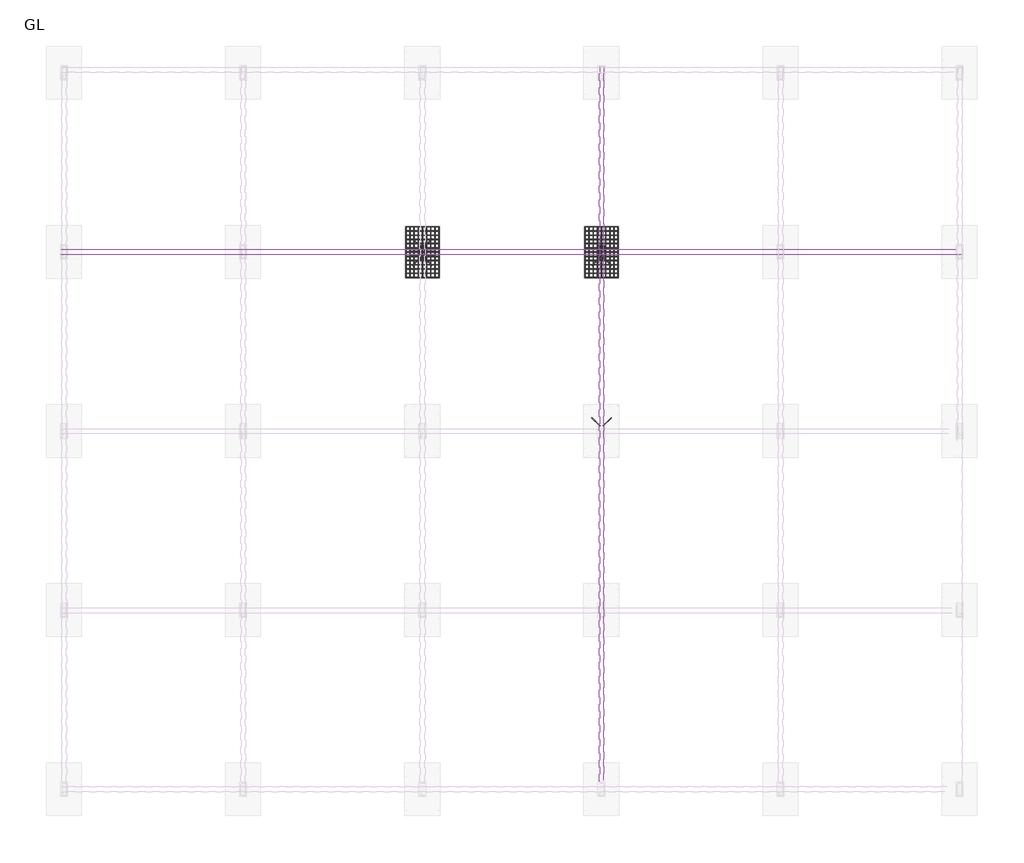
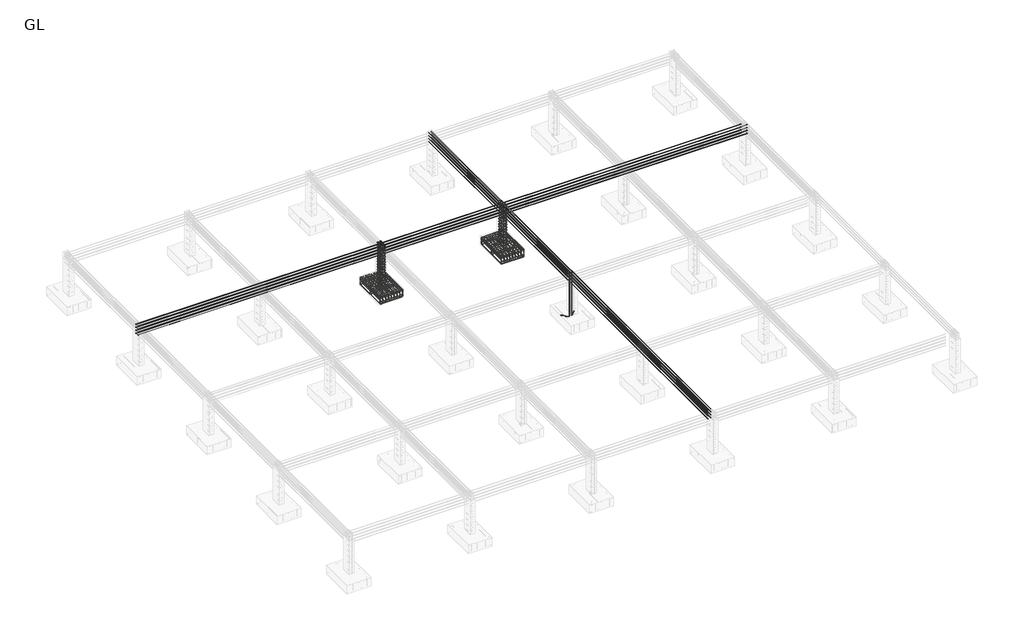
# One storey, part 9 of 16: 24 reinforcing bars.
"""IFC4 building model written with IfcOpenShell, lengths in millimetres."""

from ifc_helpers import new_model, si_unit, point, frame, origin, place, context, project, spatial, polyline, circle_curve, trimmed, segment, composite_curve, source, transform, mapped, element, save
from ifc_brep_helpers import swept_disk

model = new_model("IFC4")

# Units and contexts
model_context = context("Model", 3, world=origin())
ifc_project = project(units=[si_unit("LENGTHUNIT", "METRE", prefix="MILLI")], contexts=[model_context])

# Site, building, storey
site = spatial("IfcSite", under=ifc_project)
building = spatial("IfcBuilding", under=site)
storey = spatial("IfcBuildingStorey", under=building, Name="GL", Elevation=-1829.0)

# Reinforcing bars
placement = place(None, origin())
reinforcing_bar_shape = source(origin(), model_context, "Body", "SolidModel", [
    swept_disk(composite_curve([segment(polyline([(-3954.9544379, -1127.1167521, -2089.0), (-3954.9544379, -1127.1167521, -2213.0)]), True, "CONTINUOUS"), segment(trimmed(circle_curve(frame((-3984.9544379, -1127.1167521, -2213.0), z_axis=(0.0, 1.0, 0.0), x_axis=(30.0, 0.0, 0.0)), 30.0), [point((-3954.9544379, -1127.1167521, -2213.0))], [point((-3984.9544379, -1127.1167521, -2243.0))], True, "CARTESIAN"), True, "CONTINUOUS"), segment(polyline([(-3984.9544379, -1127.1167521, -2243.0), (-5052.9544379, -1127.1167521, -2243.0)]), True, "CONTINUOUS"), segment(trimmed(circle_curve(frame((-5052.9544379, -1127.1167521, -2213.0), z_axis=(0.0, 1.0, 0.0), x_axis=(0.0, 0.0, -30.0)), 30.0), [point((-5052.9544379, -1127.1167521, -2243.0))], [point((-5082.9544379, -1127.1167521, -2213.0))], True, "CARTESIAN"), True, "CONTINUOUS"), segment(polyline([(-5082.9544379, -1127.1167521, -2213.0), (-5082.9544379, -1127.1167521, -2089.0)]), True, "CONTINUOUS")], self_intersect=False), 6.0),
])
element("IfcReinforcingBar", 1, at=placement, inside=storey, context=model_context, shape_type="MappedRepresentation", body=[
    mapped(reinforcing_bar_shape, transform((0.0, 0.0, 0.0), x_axis=(1.0, 0.0, 0.0), y_axis=(0.0, 1.0, 0.0), z_axis=(0.0, 0.0, 1.0))),
    mapped(reinforcing_bar_shape, transform((0.0, -864.0, 0.0), x_axis=(1.0, 0.0, 0.0), y_axis=(0.0, 1.0, 0.0), z_axis=(0.0, 0.0, 1.0))),
    mapped(reinforcing_bar_shape, transform((0.0, -1728.0, 0.0), x_axis=(1.0, 0.0, 0.0), y_axis=(0.0, 1.0, 0.0), z_axis=(0.0, 0.0, 1.0))),
])
reinforcing_bar_2_shape = source(origin(), model_context, "Body", "SolidModel", [
    swept_disk(composite_curve([segment(polyline([(-5082.9544379, -1127.1167521, -2022.436678), (-5082.9544379, -1127.1167521, -1898.436678)]), True, "CONTINUOUS"), segment(trimmed(circle_curve(frame((-5052.9544379, -1127.1167521, -1898.436678), z_axis=(0.0, 1.0, 0.0), x_axis=(-30.0, 0.0, 0.0)), 30.0), [point((-5082.9544379, -1127.1167521, -1898.436678))], [point((-5052.9544379, -1127.1167521, -1868.436678))], True, "CARTESIAN"), True, "CONTINUOUS"), segment(polyline([(-5052.9544379, -1127.1167521, -1868.436678), (-3984.9544379, -1127.1167521, -1868.436678)]), True, "CONTINUOUS"), segment(trimmed(circle_curve(frame((-3984.9544379, -1127.1167521, -1898.436678), z_axis=(0.0, 1.0, 0.0), x_axis=(0.0, 0.0, 30.0)), 30.0), [point((-3984.9544379, -1127.1167521, -1868.436678))], [point((-3954.9544379, -1127.1167521, -1898.436678))], True, "CARTESIAN"), True, "CONTINUOUS"), segment(polyline([(-3954.9544379, -1127.1167521, -1898.436678), (-3954.9544379, -1127.1167521, -2022.436678)]), True, "CONTINUOUS")], self_intersect=False), 6.0),
])
element("IfcReinforcingBar", 2, at=placement, inside=storey, context=model_context, shape_type="MappedRepresentation", body=[
    mapped(reinforcing_bar_2_shape, transform((0.0, 0.0, 0.0), x_axis=(1.0, 0.0, 0.0), y_axis=(0.0, 1.0, 0.0), z_axis=(0.0, 0.0, 1.0))),
    mapped(reinforcing_bar_2_shape, transform((0.0, -144.0, 0.0), x_axis=(1.0, 0.0, 0.0), y_axis=(0.0, 1.0, 0.0), z_axis=(0.0, 0.0, 1.0))),
    mapped(reinforcing_bar_2_shape, transform((0.0, -288.0, 0.0), x_axis=(1.0, 0.0, 0.0), y_axis=(0.0, 1.0, 0.0), z_axis=(0.0, 0.0, 1.0))),
    mapped(reinforcing_bar_2_shape, transform((0.0, -432.0, 0.0), x_axis=(1.0, 0.0, 0.0), y_axis=(0.0, 1.0, 0.0), z_axis=(0.0, 0.0, 1.0))),
    mapped(reinforcing_bar_2_shape, transform((0.0, -576.0, 0.0), x_axis=(1.0, 0.0, 0.0), y_axis=(0.0, 1.0, 0.0), z_axis=(0.0, 0.0, 1.0))),
    mapped(reinforcing_bar_2_shape, transform((0.0, -720.0, 0.0), x_axis=(1.0, 0.0, 0.0), y_axis=(0.0, 1.0, 0.0), z_axis=(0.0, 0.0, 1.0))),
    mapped(reinforcing_bar_2_shape, transform((0.0, -864.0, 0.0), x_axis=(1.0, 0.0, 0.0), y_axis=(0.0, 1.0, 0.0), z_axis=(0.0, 0.0, 1.0))),
    mapped(reinforcing_bar_2_shape, transform((0.0, -1008.0, 0.0), x_axis=(1.0, 0.0, 0.0), y_axis=(0.0, 1.0, 0.0), z_axis=(0.0, 0.0, 1.0))),
    mapped(reinforcing_bar_2_shape, transform((0.0, -1152.0, 0.0), x_axis=(1.0, 0.0, 0.0), y_axis=(0.0, 1.0, 0.0), z_axis=(0.0, 0.0, 1.0))),
    mapped(reinforcing_bar_2_shape, transform((0.0, -1296.0, 0.0), x_axis=(1.0, 0.0, 0.0), y_axis=(0.0, 1.0, 0.0), z_axis=(0.0, 0.0, 1.0))),
    mapped(reinforcing_bar_2_shape, transform((0.0, -1440.0, 0.0), x_axis=(1.0, 0.0, 0.0), y_axis=(0.0, 1.0, 0.0), z_axis=(0.0, 0.0, 1.0))),
    mapped(reinforcing_bar_2_shape, transform((0.0, -1584.0, 0.0), x_axis=(1.0, 0.0, 0.0), y_axis=(0.0, 1.0, 0.0), z_axis=(0.0, 0.0, 1.0))),
    mapped(reinforcing_bar_2_shape, transform((0.0, -1728.0, 0.0), x_axis=(1.0, 0.0, 0.0), y_axis=(0.0, 1.0, 0.0), z_axis=(0.0, 0.0, 1.0))),
])
reinforcing_bar_3_shape = source(origin(), model_context, "Body", "SolidModel", [
    swept_disk(composite_curve([segment(polyline([(-5082.9544379, -2855.1167521, -2027.5081232), (-5082.9544379, -2855.1167521, -1903.5081232)]), True, "CONTINUOUS"), segment(trimmed(circle_curve(frame((-5082.9544379, -2825.1167521, -1903.5081232), z_axis=(-1.0, 0.0, 0.0), x_axis=(0.0, -30.0, 0.0)), 30.0), [point((-5082.9544379, -2855.1167521, -1903.5081232))], [point((-5082.9544379, -2825.1167521, -1873.5081232))], True, "CARTESIAN"), True, "CONTINUOUS"), segment(polyline([(-5082.9544379, -2825.1167521, -1873.5081232), (-5082.9544379, -1157.1167521, -1873.5081232)]), True, "CONTINUOUS"), segment(trimmed(circle_curve(frame((-5082.9544379, -1157.1167521, -1903.5081232), z_axis=(-1.0, 0.0, 0.0), x_axis=(0.0, 0.0, 30.0)), 30.0), [point((-5082.9544379, -1157.1167521, -1873.5081232))], [point((-5082.9544379, -1127.1167521, -1903.5081232))], True, "CARTESIAN"), True, "CONTINUOUS"), segment(polyline([(-5082.9544379, -1127.1167521, -1903.5081232), (-5082.9544379, -1127.1167521, -2027.5081232)]), True, "CONTINUOUS")], self_intersect=False), 6.0),
])
element("IfcReinforcingBar", 3, at=placement, inside=storey, context=model_context, shape_type="MappedRepresentation", body=[
    mapped(reinforcing_bar_3_shape, transform((0.0, 0.0, 0.0), x_axis=(1.0, 0.0, 0.0), y_axis=(0.0, 1.0, 0.0), z_axis=(0.0, 0.0, 1.0))),
    mapped(reinforcing_bar_3_shape, transform((141.0, 0.0, 0.0), x_axis=(1.0, 0.0, 0.0), y_axis=(0.0, 1.0, 0.0), z_axis=(0.0, 0.0, 1.0))),
    mapped(reinforcing_bar_3_shape, transform((282.0, 0.0, 0.0), x_axis=(1.0, 0.0, 0.0), y_axis=(0.0, 1.0, 0.0), z_axis=(0.0, 0.0, 1.0))),
    mapped(reinforcing_bar_3_shape, transform((423.0, 0.0, 0.0), x_axis=(1.0, 0.0, 0.0), y_axis=(0.0, 1.0, 0.0), z_axis=(0.0, 0.0, 1.0))),
    mapped(reinforcing_bar_3_shape, transform((564.0, 0.0, 0.0), x_axis=(1.0, 0.0, 0.0), y_axis=(0.0, 1.0, 0.0), z_axis=(0.0, 0.0, 1.0))),
    mapped(reinforcing_bar_3_shape, transform((705.0, 0.0, 0.0), x_axis=(1.0, 0.0, 0.0), y_axis=(0.0, 1.0, 0.0), z_axis=(0.0, 0.0, 1.0))),
    mapped(reinforcing_bar_3_shape, transform((846.0, 0.0, 0.0), x_axis=(1.0, 0.0, 0.0), y_axis=(0.0, 1.0, 0.0), z_axis=(0.0, 0.0, 1.0))),
    mapped(reinforcing_bar_3_shape, transform((987.0, 0.0, 0.0), x_axis=(1.0, 0.0, 0.0), y_axis=(0.0, 1.0, 0.0), z_axis=(0.0, 0.0, 1.0))),
    mapped(reinforcing_bar_3_shape, transform((1128.0, 0.0, 0.0), x_axis=(1.0, 0.0, 0.0), y_axis=(0.0, 1.0, 0.0), z_axis=(0.0, 0.0, 1.0))),
])
reinforcing_bar_4_shape = source(origin(), model_context, "Body", "SolidModel", [
    swept_disk(composite_curve([segment(polyline([(-3954.9544379, -2855.1167521, -2080.6239909), (-3954.9544379, -2855.1167521, -2204.6239909)]), True, "CONTINUOUS"), segment(trimmed(circle_curve(frame((-3954.9544379, -2825.1167521, -2204.6239909), z_axis=(1.0, 0.0, 0.0), x_axis=(0.0, -30.0, 0.0)), 30.0), [point((-3954.9544379, -2855.1167521, -2204.6239909))], [point((-3954.9544379, -2825.1167521, -2234.6239909))], True, "CARTESIAN"), True, "CONTINUOUS"), segment(polyline([(-3954.9544379, -2825.1167521, -2234.6239909), (-3954.9544379, -1170.1421892, -2234.6239909)]), True, "CONTINUOUS"), segment(trimmed(circle_curve(frame((-3954.9544379, -1170.1421892, -2204.6239909), z_axis=(1.0, 0.0, 0.0), x_axis=(0.0, 0.0, -30.0)), 30.0), [point((-3954.9544379, -1170.1421892, -2234.6239909))], [point((-3954.9544379, -1140.1421892, -2204.6239909))], True, "CARTESIAN"), True, "CONTINUOUS"), segment(polyline([(-3954.9544379, -1140.1421892, -2204.6239909), (-3954.9544379, -1140.1421892, -2080.6239909)]), True, "CONTINUOUS")], self_intersect=False), 6.0),
])
element("IfcReinforcingBar", 4, at=placement, inside=storey, context=model_context, shape_type="MappedRepresentation", body=[
    mapped(reinforcing_bar_4_shape, transform((0.0, 0.0, 0.0), x_axis=(1.0, 0.0, 0.0), y_axis=(0.0, 1.0, 0.0), z_axis=(0.0, 0.0, 1.0))),
    mapped(reinforcing_bar_4_shape, transform((-141.0, 0.0, 0.0), x_axis=(1.0, 0.0, 0.0), y_axis=(0.0, 1.0, 0.0), z_axis=(0.0, 0.0, 1.0))),
    mapped(reinforcing_bar_4_shape, transform((-282.0, 0.0, 0.0), x_axis=(1.0, 0.0, 0.0), y_axis=(0.0, 1.0, 0.0), z_axis=(0.0, 0.0, 1.0))),
    mapped(reinforcing_bar_4_shape, transform((-423.0, 0.0, 0.0), x_axis=(1.0, 0.0, 0.0), y_axis=(0.0, 1.0, 0.0), z_axis=(0.0, 0.0, 1.0))),
    mapped(reinforcing_bar_4_shape, transform((-564.0, 0.0, 0.0), x_axis=(1.0, 0.0, 0.0), y_axis=(0.0, 1.0, 0.0), z_axis=(0.0, 0.0, 1.0))),
    mapped(reinforcing_bar_4_shape, transform((-705.0, 0.0, 0.0), x_axis=(1.0, 0.0, 0.0), y_axis=(0.0, 1.0, 0.0), z_axis=(0.0, 0.0, 1.0))),
    mapped(reinforcing_bar_4_shape, transform((-846.0, 0.0, 0.0), x_axis=(1.0, 0.0, 0.0), y_axis=(0.0, 1.0, 0.0), z_axis=(0.0, 0.0, 1.0))),
    mapped(reinforcing_bar_4_shape, transform((-987.0, 0.0, 0.0), x_axis=(1.0, 0.0, 0.0), y_axis=(0.0, 1.0, 0.0), z_axis=(0.0, 0.0, 1.0))),
    mapped(reinforcing_bar_4_shape, transform((-1128.0, 0.0, 0.0), x_axis=(1.0, 0.0, 0.0), y_axis=(0.0, 1.0, 0.0), z_axis=(0.0, 0.0, 1.0))),
])
reinforcing_bar_5_shape = source(origin(), model_context, "Body", "SolidModel", [
    swept_disk(composite_curve([segment(polyline([(-10050.9544379, -1127.1167521, -2089.0), (-10050.9544379, -1127.1167521, -2213.0)]), True, "CONTINUOUS"), segment(trimmed(circle_curve(frame((-10080.9544379, -1127.1167521, -2213.0), z_axis=(0.0, 1.0, 0.0), x_axis=(30.0, 0.0, 0.0)), 30.0), [point((-10050.9544379, -1127.1167521, -2213.0))], [point((-10080.9544379, -1127.1167521, -2243.0))], True, "CARTESIAN"), True, "CONTINUOUS"), segment(polyline([(-10080.9544379, -1127.1167521, -2243.0), (-11148.9544379, -1127.1167521, -2243.0)]), True, "CONTINUOUS"), segment(trimmed(circle_curve(frame((-11148.9544379, -1127.1167521, -2213.0), z_axis=(0.0, 1.0, 0.0), x_axis=(0.0, 0.0, -30.0)), 30.0), [point((-11148.9544379, -1127.1167521, -2243.0))], [point((-11178.9544379, -1127.1167521, -2213.0))], True, "CARTESIAN"), True, "CONTINUOUS"), segment(polyline([(-11178.9544379, -1127.1167521, -2213.0), (-11178.9544379, -1127.1167521, -2089.0)]), True, "CONTINUOUS")], self_intersect=False), 6.0),
])
element("IfcReinforcingBar", 5, at=placement, inside=storey, context=model_context, shape_type="MappedRepresentation", body=[
    mapped(reinforcing_bar_5_shape, transform((0.0, 0.0, 0.0), x_axis=(1.0, 0.0, 0.0), y_axis=(0.0, 1.0, 0.0), z_axis=(0.0, 0.0, 1.0))),
    mapped(reinforcing_bar_5_shape, transform((0.0, -864.0, 0.0), x_axis=(1.0, 0.0, 0.0), y_axis=(0.0, 1.0, 0.0), z_axis=(0.0, 0.0, 1.0))),
    mapped(reinforcing_bar_5_shape, transform((0.0, -1728.0, 0.0), x_axis=(1.0, 0.0, 0.0), y_axis=(0.0, 1.0, 0.0), z_axis=(0.0, 0.0, 1.0))),
])
reinforcing_bar_6_shape = source(origin(), model_context, "Body", "SolidModel", [
    swept_disk(composite_curve([segment(polyline([(-11178.9544379, -1127.1167521, -2022.436678), (-11178.9544379, -1127.1167521, -1898.436678)]), True, "CONTINUOUS"), segment(trimmed(circle_curve(frame((-11148.9544379, -1127.1167521, -1898.436678), z_axis=(0.0, 1.0, 0.0), x_axis=(-30.0, 0.0, 0.0)), 30.0), [point((-11178.9544379, -1127.1167521, -1898.436678))], [point((-11148.9544379, -1127.1167521, -1868.436678))], True, "CARTESIAN"), True, "CONTINUOUS"), segment(polyline([(-11148.9544379, -1127.1167521, -1868.436678), (-10080.9544379, -1127.1167521, -1868.436678)]), True, "CONTINUOUS"), segment(trimmed(circle_curve(frame((-10080.9544379, -1127.1167521, -1898.436678), z_axis=(0.0, 1.0, 0.0), x_axis=(0.0, 0.0, 30.0)), 30.0), [point((-10080.9544379, -1127.1167521, -1868.436678))], [point((-10050.9544379, -1127.1167521, -1898.436678))], True, "CARTESIAN"), True, "CONTINUOUS"), segment(polyline([(-10050.9544379, -1127.1167521, -1898.436678), (-10050.9544379, -1127.1167521, -2022.436678)]), True, "CONTINUOUS")], self_intersect=False), 6.0),
])
element("IfcReinforcingBar", 6, at=placement, inside=storey, context=model_context, shape_type="MappedRepresentation", body=[
    mapped(reinforcing_bar_6_shape, transform((0.0, 0.0, 0.0), x_axis=(1.0, 0.0, 0.0), y_axis=(0.0, 1.0, 0.0), z_axis=(0.0, 0.0, 1.0))),
    mapped(reinforcing_bar_6_shape, transform((0.0, -144.0, 0.0), x_axis=(1.0, 0.0, 0.0), y_axis=(0.0, 1.0, 0.0), z_axis=(0.0, 0.0, 1.0))),
    mapped(reinforcing_bar_6_shape, transform((0.0, -288.0, 0.0), x_axis=(1.0, 0.0, 0.0), y_axis=(0.0, 1.0, 0.0), z_axis=(0.0, 0.0, 1.0))),
    mapped(reinforcing_bar_6_shape, transform((0.0, -432.0, 0.0), x_axis=(1.0, 0.0, 0.0), y_axis=(0.0, 1.0, 0.0), z_axis=(0.0, 0.0, 1.0))),
    mapped(reinforcing_bar_6_shape, transform((0.0, -576.0, 0.0), x_axis=(1.0, 0.0, 0.0), y_axis=(0.0, 1.0, 0.0), z_axis=(0.0, 0.0, 1.0))),
    mapped(reinforcing_bar_6_shape, transform((0.0, -720.0, 0.0), x_axis=(1.0, 0.0, 0.0), y_axis=(0.0, 1.0, 0.0), z_axis=(0.0, 0.0, 1.0))),
    mapped(reinforcing_bar_6_shape, transform((0.0, -864.0, 0.0), x_axis=(1.0, 0.0, 0.0), y_axis=(0.0, 1.0, 0.0), z_axis=(0.0, 0.0, 1.0))),
    mapped(reinforcing_bar_6_shape, transform((0.0, -1008.0, 0.0), x_axis=(1.0, 0.0, 0.0), y_axis=(0.0, 1.0, 0.0), z_axis=(0.0, 0.0, 1.0))),
    mapped(reinforcing_bar_6_shape, transform((0.0, -1152.0, 0.0), x_axis=(1.0, 0.0, 0.0), y_axis=(0.0, 1.0, 0.0), z_axis=(0.0, 0.0, 1.0))),
    mapped(reinforcing_bar_6_shape, transform((0.0, -1296.0, 0.0), x_axis=(1.0, 0.0, 0.0), y_axis=(0.0, 1.0, 0.0), z_axis=(0.0, 0.0, 1.0))),
    mapped(reinforcing_bar_6_shape, transform((0.0, -1440.0, 0.0), x_axis=(1.0, 0.0, 0.0), y_axis=(0.0, 1.0, 0.0), z_axis=(0.0, 0.0, 1.0))),
    mapped(reinforcing_bar_6_shape, transform((0.0, -1584.0, 0.0), x_axis=(1.0, 0.0, 0.0), y_axis=(0.0, 1.0, 0.0), z_axis=(0.0, 0.0, 1.0))),
    mapped(reinforcing_bar_6_shape, transform((0.0, -1728.0, 0.0), x_axis=(1.0, 0.0, 0.0), y_axis=(0.0, 1.0, 0.0), z_axis=(0.0, 0.0, 1.0))),
])
reinforcing_bar_7_shape = source(origin(), model_context, "Body", "SolidModel", [
    swept_disk(composite_curve([segment(polyline([(-11178.9544379, -2855.1167521, -2027.5081232), (-11178.9544379, -2855.1167521, -1903.5081232)]), True, "CONTINUOUS"), segment(trimmed(circle_curve(frame((-11178.9544379, -2825.1167521, -1903.5081232), z_axis=(-1.0, 0.0, 0.0), x_axis=(0.0, -30.0, 0.0)), 30.0), [point((-11178.9544379, -2855.1167521, -1903.5081232))], [point((-11178.9544379, -2825.1167521, -1873.5081232))], True, "CARTESIAN"), True, "CONTINUOUS"), segment(polyline([(-11178.9544379, -2825.1167521, -1873.5081232), (-11178.9544379, -1157.1167521, -1873.5081232)]), True, "CONTINUOUS"), segment(trimmed(circle_curve(frame((-11178.9544379, -1157.1167521, -1903.5081232), z_axis=(-1.0, 0.0, 0.0), x_axis=(0.0, 0.0, 30.0)), 30.0), [point((-11178.9544379, -1157.1167521, -1873.5081232))], [point((-11178.9544379, -1127.1167521, -1903.5081232))], True, "CARTESIAN"), True, "CONTINUOUS"), segment(polyline([(-11178.9544379, -1127.1167521, -1903.5081232), (-11178.9544379, -1127.1167521, -2027.5081232)]), True, "CONTINUOUS")], self_intersect=False), 6.0),
])
element("IfcReinforcingBar", 7, at=placement, inside=storey, context=model_context, shape_type="MappedRepresentation", body=[
    mapped(reinforcing_bar_7_shape, transform((0.0, 0.0, 0.0), x_axis=(1.0, 0.0, 0.0), y_axis=(0.0, 1.0, 0.0), z_axis=(0.0, 0.0, 1.0))),
    mapped(reinforcing_bar_7_shape, transform((141.0, 0.0, 0.0), x_axis=(1.0, 0.0, 0.0), y_axis=(0.0, 1.0, 0.0), z_axis=(0.0, 0.0, 1.0))),
    mapped(reinforcing_bar_7_shape, transform((282.0, 0.0, 0.0), x_axis=(1.0, 0.0, 0.0), y_axis=(0.0, 1.0, 0.0), z_axis=(0.0, 0.0, 1.0))),
    mapped(reinforcing_bar_7_shape, transform((423.0, 0.0, 0.0), x_axis=(1.0, 0.0, 0.0), y_axis=(0.0, 1.0, 0.0), z_axis=(0.0, 0.0, 1.0))),
    mapped(reinforcing_bar_7_shape, transform((564.0, 0.0, 0.0), x_axis=(1.0, 0.0, 0.0), y_axis=(0.0, 1.0, 0.0), z_axis=(0.0, 0.0, 1.0))),
    mapped(reinforcing_bar_7_shape, transform((705.0, 0.0, 0.0), x_axis=(1.0, 0.0, 0.0), y_axis=(0.0, 1.0, 0.0), z_axis=(0.0, 0.0, 1.0))),
    mapped(reinforcing_bar_7_shape, transform((846.0, 0.0, 0.0), x_axis=(1.0, 0.0, 0.0), y_axis=(0.0, 1.0, 0.0), z_axis=(0.0, 0.0, 1.0))),
    mapped(reinforcing_bar_7_shape, transform((987.0, 0.0, 0.0), x_axis=(1.0, 0.0, 0.0), y_axis=(0.0, 1.0, 0.0), z_axis=(0.0, 0.0, 1.0))),
    mapped(reinforcing_bar_7_shape, transform((1128.0, 0.0, 0.0), x_axis=(1.0, 0.0, 0.0), y_axis=(0.0, 1.0, 0.0), z_axis=(0.0, 0.0, 1.0))),
])
reinforcing_bar_8_shape = source(origin(), model_context, "Body", "SolidModel", [
    swept_disk(composite_curve([segment(polyline([(-10050.9544379, -2855.1167521, -2080.6239909), (-10050.9544379, -2855.1167521, -2204.6239909)]), True, "CONTINUOUS"), segment(trimmed(circle_curve(frame((-10050.9544379, -2825.1167521, -2204.6239909), z_axis=(1.0, 0.0, 0.0), x_axis=(0.0, -30.0, 0.0)), 30.0), [point((-10050.9544379, -2855.1167521, -2204.6239909))], [point((-10050.9544379, -2825.1167521, -2234.6239909))], True, "CARTESIAN"), True, "CONTINUOUS"), segment(polyline([(-10050.9544379, -2825.1167521, -2234.6239909), (-10050.9544379, -1170.1421892, -2234.6239909)]), True, "CONTINUOUS"), segment(trimmed(circle_curve(frame((-10050.9544379, -1170.1421892, -2204.6239909), z_axis=(1.0, 0.0, 0.0), x_axis=(0.0, 0.0, -30.0)), 30.0), [point((-10050.9544379, -1170.1421892, -2234.6239909))], [point((-10050.9544379, -1140.1421892, -2204.6239909))], True, "CARTESIAN"), True, "CONTINUOUS"), segment(polyline([(-10050.9544379, -1140.1421892, -2204.6239909), (-10050.9544379, -1140.1421892, -2080.6239909)]), True, "CONTINUOUS")], self_intersect=False), 6.0),
])
element("IfcReinforcingBar", 8, at=placement, inside=storey, context=model_context, shape_type="MappedRepresentation", body=[
    mapped(reinforcing_bar_8_shape, transform((0.0, 0.0, 0.0), x_axis=(1.0, 0.0, 0.0), y_axis=(0.0, 1.0, 0.0), z_axis=(0.0, 0.0, 1.0))),
    mapped(reinforcing_bar_8_shape, transform((-141.0, 0.0, 0.0), x_axis=(1.0, 0.0, 0.0), y_axis=(0.0, 1.0, 0.0), z_axis=(0.0, 0.0, 1.0))),
    mapped(reinforcing_bar_8_shape, transform((-282.0, 0.0, 0.0), x_axis=(1.0, 0.0, 0.0), y_axis=(0.0, 1.0, 0.0), z_axis=(0.0, 0.0, 1.0))),
    mapped(reinforcing_bar_8_shape, transform((-423.0, 0.0, 0.0), x_axis=(1.0, 0.0, 0.0), y_axis=(0.0, 1.0, 0.0), z_axis=(0.0, 0.0, 1.0))),
    mapped(reinforcing_bar_8_shape, transform((-564.0, 0.0, 0.0), x_axis=(1.0, 0.0, 0.0), y_axis=(0.0, 1.0, 0.0), z_axis=(0.0, 0.0, 1.0))),
    mapped(reinforcing_bar_8_shape, transform((-705.0, 0.0, 0.0), x_axis=(1.0, 0.0, 0.0), y_axis=(0.0, 1.0, 0.0), z_axis=(0.0, 0.0, 1.0))),
    mapped(reinforcing_bar_8_shape, transform((-846.0, 0.0, 0.0), x_axis=(1.0, 0.0, 0.0), y_axis=(0.0, 1.0, 0.0), z_axis=(0.0, 0.0, 1.0))),
    mapped(reinforcing_bar_8_shape, transform((-987.0, 0.0, 0.0), x_axis=(1.0, 0.0, 0.0), y_axis=(0.0, 1.0, 0.0), z_axis=(0.0, 0.0, 1.0))),
    mapped(reinforcing_bar_8_shape, transform((-1128.0, 0.0, 0.0), x_axis=(1.0, 0.0, 0.0), y_axis=(0.0, 1.0, 0.0), z_axis=(0.0, 0.0, 1.0))),
])
reinforcing_bar_9_shape = source(origin(), model_context, "Body", "SolidModel", [
    swept_disk(composite_curve([segment(polyline([(-10607.4864005, -2066.2223078, -1793.0), (-10695.1676414, -2153.9035486, -1793.0)]), True, "CONTINUOUS"), segment(trimmed(circle_curve(frame((-10673.9544379, -2175.1167521, -1793.0), z_axis=(0.0, 0.0, 1.0), x_axis=(-21.21320349999951, 21.213203500000418, 0.0)), 30.0), [point((-10695.1676414, -2153.9035486, -1793.0))], [point((-10673.9544379, -2205.1167521, -1793.0))], True, "CARTESIAN"), True, "CONTINUOUS"), segment(polyline([(-10673.9544379, -2205.1167521, -1793.0), (-10555.9544379, -2205.1167521, -1793.0)]), True, "CONTINUOUS"), segment(trimmed(circle_curve(frame((-10555.9544379, -2175.1167521, -1793.0), z_axis=(0.0, 0.0, 1.0), x_axis=(0.0, -30.0, 0.0)), 30.0), [point((-10555.9544379, -2205.1167521, -1793.0))], [point((-10525.9544379, -2175.1167521, -1793.0))], True, "CARTESIAN"), True, "CONTINUOUS"), segment(polyline([(-10525.9544379, -2175.1167521, -1793.0), (-10525.9544379, -1807.1167521, -1793.0)]), True, "CONTINUOUS"), segment(trimmed(circle_curve(frame((-10555.8864962, -1807.1167521, -1795.0178916), z_axis=(-0.06726305234213417, 0.0, 0.9977352764083365), x_axis=(29.93205830000079, 0.0, 2.0178915999999845)), 30.0), [point((-10525.9544379, -1807.1167521, -1793.0))], [point((-10555.8864962, -1777.1167521, -1795.0178916))], True, "CARTESIAN"), True, "CONTINUOUS"), segment(polyline([(-10555.8864962, -1777.1167521, -1795.0178916), (-10674.0223796, -1777.1167521, -1802.9821084)]), True, "CONTINUOUS"), segment(trimmed(circle_curve(frame((-10674.0223796, -1807.1167521, -1802.9821084), z_axis=(-0.06726305234213417, 0.0, 0.9977352764083365), x_axis=(0.0, 30.0, 0.0)), 30.0), [point((-10674.0223796, -1777.1167521, -1802.9821084))], [point((-10703.9544379, -1807.1167521, -1805.0))], True, "CARTESIAN"), True, "CONTINUOUS"), segment(polyline([(-10703.9544379, -1807.1167521, -1805.0), (-10703.9544379, -2175.1167521, -1805.0)]), True, "CONTINUOUS"), segment(trimmed(circle_curve(frame((-10673.9544379, -2175.1167521, -1805.0), z_axis=(0.0, 0.0, 1.0), x_axis=(-30.0, 0.0, 0.0)), 30.0), [point((-10703.9544379, -2175.1167521, -1805.0))], [point((-10652.7412345, -2196.3299555, -1805.0))], True, "CARTESIAN"), True, "CONTINUOUS"), segment(polyline([(-10652.7412345, -2196.3299555, -1805.0), (-10565.0599936, -2108.6487146, -1805.0)]), True, "CONTINUOUS")], self_intersect=False), 6.0),
])
element("IfcReinforcingBar", 9, at=placement, inside=storey, context=model_context, shape_type="MappedRepresentation", body=[
    mapped(reinforcing_bar_9_shape, transform((0.0, 0.0, 0.0), x_axis=(1.0, 0.0, 0.0), y_axis=(0.0, 1.0, 0.0), z_axis=(0.0, 0.0, 1.0))),
    mapped(reinforcing_bar_9_shape, transform((0.0, 0.0, 144.8571429), x_axis=(1.0, 0.0, 0.0), y_axis=(0.0, 1.0, 0.0), z_axis=(0.0, 0.0, 1.0))),
    mapped(reinforcing_bar_9_shape, transform((0.0, 0.0, 289.7142857), x_axis=(1.0, 0.0, 0.0), y_axis=(0.0, 1.0, 0.0), z_axis=(0.0, 0.0, 1.0))),
    mapped(reinforcing_bar_9_shape, transform((0.0, 0.0, 434.5714286), x_axis=(1.0, 0.0, 0.0), y_axis=(0.0, 1.0, 0.0), z_axis=(0.0, 0.0, 1.0))),
    mapped(reinforcing_bar_9_shape, transform((0.0, 0.0, 579.4285714), x_axis=(1.0, 0.0, 0.0), y_axis=(0.0, 1.0, 0.0), z_axis=(0.0, 0.0, 1.0))),
    mapped(reinforcing_bar_9_shape, transform((0.0, 0.0, 724.2857143), x_axis=(1.0, 0.0, 0.0), y_axis=(0.0, 1.0, 0.0), z_axis=(0.0, 0.0, 1.0))),
    mapped(reinforcing_bar_9_shape, transform((0.0, 0.0, 869.1428571), x_axis=(1.0, 0.0, 0.0), y_axis=(0.0, 1.0, 0.0), z_axis=(0.0, 0.0, 1.0))),
    mapped(reinforcing_bar_9_shape, transform((0.0, 0.0, 1014.0), x_axis=(1.0, 0.0, 0.0), y_axis=(0.0, 1.0, 0.0), z_axis=(0.0, 0.0, 1.0))),
    mapped(reinforcing_bar_9_shape, transform((0.0, 0.0, 1158.8571429), x_axis=(1.0, 0.0, 0.0), y_axis=(0.0, 1.0, 0.0), z_axis=(0.0, 0.0, 1.0))),
    mapped(reinforcing_bar_9_shape, transform((0.0, 0.0, 1303.7142857), x_axis=(1.0, 0.0, 0.0), y_axis=(0.0, 1.0, 0.0), z_axis=(0.0, 0.0, 1.0))),
    mapped(reinforcing_bar_9_shape, transform((0.0, 0.0, 1448.5714286), x_axis=(1.0, 0.0, 0.0), y_axis=(0.0, 1.0, 0.0), z_axis=(0.0, 0.0, 1.0))),
    mapped(reinforcing_bar_9_shape, transform((0.0, 0.0, 1593.4285714), x_axis=(1.0, 0.0, 0.0), y_axis=(0.0, 1.0, 0.0), z_axis=(0.0, 0.0, 1.0))),
    mapped(reinforcing_bar_9_shape, transform((0.0, 0.0, 1738.2857143), x_axis=(1.0, 0.0, 0.0), y_axis=(0.0, 1.0, 0.0), z_axis=(0.0, 0.0, 1.0))),
    mapped(reinforcing_bar_9_shape, transform((0.0, 0.0, 1883.1428571), x_axis=(1.0, 0.0, 0.0), y_axis=(0.0, 1.0, 0.0), z_axis=(0.0, 0.0, 1.0))),
    mapped(reinforcing_bar_9_shape, transform((0.0, 0.0, 2028.0), x_axis=(1.0, 0.0, 0.0), y_axis=(0.0, 1.0, 0.0), z_axis=(0.0, 0.0, 1.0))),
])
element("IfcReinforcingBar", 10, at=placement, inside=storey, context=model_context, shape_type="SolidModel", body=[
    swept_disk(composite_curve([segment(polyline([(-10672.0642232, -2176.0642439, 241.0), (-10672.0642232, -2176.0642439, -2129.0)]), True, "CONTINUOUS"), segment(trimmed(circle_curve(frame((-10693.2774266, -2197.2774473, -2129.0), z_axis=(-0.7071067811865187, 0.7071067811865764, 0.0), x_axis=(21.213203400000566, 21.21320340000011, 0.0)), 30.0), [point((-10672.0642232, -2176.0642439, -2129.0))], [point((-10693.2774266, -2197.2774473, -2159.0))], True, "CARTESIAN"), True, "CONTINUOUS"), segment(polyline([(-10693.2774266, -2197.2774473, -2159.0), (-10940.7648, -2444.7648207, -2159.0)]), True, "CONTINUOUS")], self_intersect=False), 6.0),
])
element("IfcReinforcingBar", 11, at=placement, inside=storey, context=model_context, shape_type="SolidModel", body=[
    swept_disk(composite_curve([segment(polyline([(-10672.0642232, -1806.1692603, 241.0), (-10672.0642232, -1806.1692603, -2129.0)]), True, "CONTINUOUS"), segment(trimmed(circle_curve(frame((-10693.2774266, -1784.9560568, -2129.0), z_axis=(0.7071067811865218, 0.7071067811865733, 0.0), x_axis=(21.213203400000566, -21.213203499999963, 0.0)), 30.0), [point((-10672.0642232, -1806.1692603, -2129.0))], [point((-10693.2774266, -1784.9560568, -2159.0))], True, "CARTESIAN"), True, "CONTINUOUS"), segment(polyline([(-10693.2774266, -1784.9560568, -2159.0), (-10940.7648, -1537.4686834, -2159.0)]), True, "CONTINUOUS")], self_intersect=False), 6.0),
])
element("IfcReinforcingBar", 12, at=placement, inside=storey, context=model_context, shape_type="SolidModel", body=[
    swept_disk(composite_curve([segment(polyline([(-10557.8446527, -2176.0642439, 241.0), (-10557.8446527, -2176.0642439, -2129.0)]), True, "CONTINUOUS"), segment(trimmed(circle_curve(frame((-10536.6314492, -2197.2774473, -2129.0), z_axis=(-0.7071067811865248, -0.7071067811865703, 0.0), x_axis=(-21.21320349999951, 21.21320340000011, 0.0)), 30.0), [point((-10557.8446527, -2176.0642439, -2129.0))], [point((-10536.6314492, -2197.2774473, -2159.0))], True, "CARTESIAN"), True, "CONTINUOUS"), segment(polyline([(-10536.6314492, -2197.2774473, -2159.0), (-10289.1440758, -2444.7648207, -2159.0)]), True, "CONTINUOUS")], self_intersect=False), 6.0),
])
element("IfcReinforcingBar", 13, at=placement, inside=storey, context=model_context, shape_type="SolidModel", body=[
    swept_disk(composite_curve([segment(polyline([(-10557.8446527, -1806.1692603, 241.0), (-10557.8446527, -1806.1692603, -2129.0)]), True, "CONTINUOUS"), segment(trimmed(circle_curve(frame((-10536.6314492, -1784.9560568, -2129.0), z_axis=(0.7071067811865157, -0.7071067811865794, 0.0), x_axis=(-21.21320349999951, -21.213203499999963, 0.0)), 30.0), [point((-10557.8446527, -1806.1692603, -2129.0))], [point((-10536.6314492, -1784.9560568, -2159.0))], True, "CARTESIAN"), True, "CONTINUOUS"), segment(polyline([(-10536.6314492, -1784.9560568, -2159.0), (-10289.1440758, -1537.4686834, -2159.0)]), True, "CONTINUOUS")], self_intersect=False), 6.0),
])
reinforcing_bar_10_shape = source(origin(), model_context, "Body", "SolidModel", [
    swept_disk(composite_curve([segment(polyline([(-10672.0642232, -2098.9117405, 241.0), (-10672.0642232, -2098.9117405, -2129.0)]), True, "CONTINUOUS"), segment(trimmed(circle_curve(frame((-10702.0642232, -2098.9117405, -2129.0), z_axis=(0.0, 1.0, 0.0), x_axis=(30.0, 0.0, 0.0)), 30.0), [point((-10672.0642232, -2098.9117405, -2129.0))], [point((-10702.0642232, -2098.9117405, -2159.0))], True, "CARTESIAN"), True, "CONTINUOUS"), segment(polyline([(-10702.0642232, -2098.9117405, -2159.0), (-11052.0642232, -2098.9117405, -2159.0)]), True, "CONTINUOUS")], self_intersect=False), 6.0),
])
element("IfcReinforcingBar", 14, at=placement, inside=storey, context=model_context, shape_type="MappedRepresentation", body=[
    mapped(reinforcing_bar_10_shape, transform((0.0, 0.0, 0.0), x_axis=(1.0, 0.0, 0.0), y_axis=(0.0, 1.0, 0.0), z_axis=(0.0, 0.0, 1.0))),
    mapped(reinforcing_bar_10_shape, transform((0.0, 123.5823926, 0.0), x_axis=(1.0, 0.0, 0.0), y_axis=(0.0, 1.0, 0.0), z_axis=(0.0, 0.0, 1.0))),
    mapped(reinforcing_bar_10_shape, transform((0.0, 247.1647853, 0.0), x_axis=(1.0, 0.0, 0.0), y_axis=(0.0, 1.0, 0.0), z_axis=(0.0, 0.0, 1.0))),
])
reinforcing_bar_11_shape = source(origin(), model_context, "Body", "SolidModel", [
    swept_disk(composite_curve([segment(polyline([(-10557.8446527, -2098.9117405, 241.0), (-10557.8446527, -2098.9117405, -2129.0)]), True, "CONTINUOUS"), segment(trimmed(circle_curve(frame((-10527.8446527, -2098.9117405, -2129.0), z_axis=(0.0, -1.0, 0.0), x_axis=(-30.0, 0.0, 0.0)), 30.0), [point((-10557.8446527, -2098.9117405, -2129.0))], [point((-10527.8446527, -2098.9117405, -2159.0))], True, "CARTESIAN"), True, "CONTINUOUS"), segment(polyline([(-10527.8446527, -2098.9117405, -2159.0), (-10177.8446527, -2098.9117405, -2159.0)]), True, "CONTINUOUS")], self_intersect=False), 6.0),
])
element("IfcReinforcingBar", 15, at=placement, inside=storey, context=model_context, shape_type="MappedRepresentation", body=[
    mapped(reinforcing_bar_11_shape, transform((0.0, 0.0, 0.0), x_axis=(1.0, 0.0, 0.0), y_axis=(0.0, 1.0, 0.0), z_axis=(0.0, 0.0, 1.0))),
    mapped(reinforcing_bar_11_shape, transform((0.0, 123.5823926, 0.0), x_axis=(1.0, 0.0, 0.0), y_axis=(0.0, 1.0, 0.0), z_axis=(0.0, 0.0, 1.0))),
    mapped(reinforcing_bar_11_shape, transform((0.0, 247.1647853, 0.0), x_axis=(1.0, 0.0, 0.0), y_axis=(0.0, 1.0, 0.0), z_axis=(0.0, 0.0, 1.0))),
])
reinforcing_bar_12_shape = source(origin(), model_context, "Body", "SolidModel", [
    swept_disk(composite_curve([segment(polyline([(-4511.4864005, -2066.2223078, -1793.0), (-4599.1676414, -2153.9035486, -1793.0)]), True, "CONTINUOUS"), segment(trimmed(circle_curve(frame((-4577.9544379, -2175.1167521, -1793.0), z_axis=(0.0, 0.0, 1.0), x_axis=(-21.213203500000418, 21.213203500000418, 0.0)), 30.0), [point((-4599.1676414, -2153.9035486, -1793.0))], [point((-4577.9544379, -2205.1167521, -1793.0))], True, "CARTESIAN"), True, "CONTINUOUS"), segment(polyline([(-4577.9544379, -2205.1167521, -1793.0), (-4459.9544379, -2205.1167521, -1793.0)]), True, "CONTINUOUS"), segment(trimmed(circle_curve(frame((-4459.9544379, -2175.1167521, -1793.0), z_axis=(0.0, 0.0, 1.0), x_axis=(0.0, -30.0, 0.0)), 30.0), [point((-4459.9544379, -2205.1167521, -1793.0))], [point((-4429.9544379, -2175.1167521, -1793.0))], True, "CARTESIAN"), True, "CONTINUOUS"), segment(polyline([(-4429.9544379, -2175.1167521, -1793.0), (-4429.9544379, -1807.1167521, -1793.0)]), True, "CONTINUOUS"), segment(trimmed(circle_curve(frame((-4459.8864962, -1807.1167521, -1795.0178916), z_axis=(-0.06726305234213417, 0.0, 0.9977352764083365), x_axis=(29.93205829999988, 0.0, 2.0178915999999845)), 30.0), [point((-4429.9544379, -1807.1167521, -1793.0))], [point((-4459.8864962, -1777.1167521, -1795.0178916))], True, "CARTESIAN"), True, "CONTINUOUS"), segment(polyline([(-4459.8864962, -1777.1167521, -1795.0178916), (-4578.0223796, -1777.1167521, -1802.9821084)]), True, "CONTINUOUS"), segment(trimmed(circle_curve(frame((-4578.0223796, -1807.1167521, -1802.9821084), z_axis=(-0.06726305234213417, 0.0, 0.9977352764083365), x_axis=(0.0, 30.0, 0.0)), 30.0), [point((-4578.0223796, -1777.1167521, -1802.9821084))], [point((-4607.9544379, -1807.1167521, -1805.0))], True, "CARTESIAN"), True, "CONTINUOUS"), segment(polyline([(-4607.9544379, -1807.1167521, -1805.0), (-4607.9544379, -2175.1167521, -1805.0)]), True, "CONTINUOUS"), segment(trimmed(circle_curve(frame((-4577.9544379, -2175.1167521, -1805.0), z_axis=(0.0, 0.0, 1.0), x_axis=(-30.0, 0.0, 0.0)), 30.0), [point((-4607.9544379, -2175.1167521, -1805.0))], [point((-4556.7412345, -2196.3299555, -1805.0))], True, "CARTESIAN"), True, "CONTINUOUS"), segment(polyline([(-4556.7412345, -2196.3299555, -1805.0), (-4469.0599936, -2108.6487146, -1805.0)]), True, "CONTINUOUS")], self_intersect=False), 6.0),
])
element("IfcReinforcingBar", 16, at=placement, inside=storey, context=model_context, shape_type="MappedRepresentation", body=[
    mapped(reinforcing_bar_12_shape, transform((0.0, 0.0, 0.0), x_axis=(1.0, 0.0, 0.0), y_axis=(0.0, 1.0, 0.0), z_axis=(0.0, 0.0, 1.0))),
    mapped(reinforcing_bar_12_shape, transform((0.0, 0.0, 144.8571429), x_axis=(1.0, 0.0, 0.0), y_axis=(0.0, 1.0, 0.0), z_axis=(0.0, 0.0, 1.0))),
    mapped(reinforcing_bar_12_shape, transform((0.0, 0.0, 289.7142857), x_axis=(1.0, 0.0, 0.0), y_axis=(0.0, 1.0, 0.0), z_axis=(0.0, 0.0, 1.0))),
    mapped(reinforcing_bar_12_shape, transform((0.0, 0.0, 434.5714286), x_axis=(1.0, 0.0, 0.0), y_axis=(0.0, 1.0, 0.0), z_axis=(0.0, 0.0, 1.0))),
    mapped(reinforcing_bar_12_shape, transform((0.0, 0.0, 579.4285714), x_axis=(1.0, 0.0, 0.0), y_axis=(0.0, 1.0, 0.0), z_axis=(0.0, 0.0, 1.0))),
    mapped(reinforcing_bar_12_shape, transform((0.0, 0.0, 724.2857143), x_axis=(1.0, 0.0, 0.0), y_axis=(0.0, 1.0, 0.0), z_axis=(0.0, 0.0, 1.0))),
    mapped(reinforcing_bar_12_shape, transform((0.0, 0.0, 869.1428571), x_axis=(1.0, 0.0, 0.0), y_axis=(0.0, 1.0, 0.0), z_axis=(0.0, 0.0, 1.0))),
    mapped(reinforcing_bar_12_shape, transform((0.0, 0.0, 1014.0), x_axis=(1.0, 0.0, 0.0), y_axis=(0.0, 1.0, 0.0), z_axis=(0.0, 0.0, 1.0))),
    mapped(reinforcing_bar_12_shape, transform((0.0, 0.0, 1158.8571429), x_axis=(1.0, 0.0, 0.0), y_axis=(0.0, 1.0, 0.0), z_axis=(0.0, 0.0, 1.0))),
    mapped(reinforcing_bar_12_shape, transform((0.0, 0.0, 1303.7142857), x_axis=(1.0, 0.0, 0.0), y_axis=(0.0, 1.0, 0.0), z_axis=(0.0, 0.0, 1.0))),
    mapped(reinforcing_bar_12_shape, transform((0.0, 0.0, 1448.5714286), x_axis=(1.0, 0.0, 0.0), y_axis=(0.0, 1.0, 0.0), z_axis=(0.0, 0.0, 1.0))),
    mapped(reinforcing_bar_12_shape, transform((0.0, 0.0, 1593.4285714), x_axis=(1.0, 0.0, 0.0), y_axis=(0.0, 1.0, 0.0), z_axis=(0.0, 0.0, 1.0))),
    mapped(reinforcing_bar_12_shape, transform((0.0, 0.0, 1738.2857143), x_axis=(1.0, 0.0, 0.0), y_axis=(0.0, 1.0, 0.0), z_axis=(0.0, 0.0, 1.0))),
    mapped(reinforcing_bar_12_shape, transform((0.0, 0.0, 1883.1428571), x_axis=(1.0, 0.0, 0.0), y_axis=(0.0, 1.0, 0.0), z_axis=(0.0, 0.0, 1.0))),
    mapped(reinforcing_bar_12_shape, transform((0.0, 0.0, 2028.0), x_axis=(1.0, 0.0, 0.0), y_axis=(0.0, 1.0, 0.0), z_axis=(0.0, 0.0, 1.0))),
])
element("IfcReinforcingBar", 17, at=placement, inside=storey, context=model_context, shape_type="SolidModel", body=[
    swept_disk(composite_curve([segment(polyline([(-4576.0642232, -2176.0642439, 241.0), (-4576.0642232, -2176.0642439, -2129.0)]), True, "CONTINUOUS"), segment(trimmed(circle_curve(frame((-4597.2774266, -2197.2774473, -2129.0), z_axis=(-0.7071067811865187, 0.7071067811865764, 0.0), x_axis=(21.213203399999657, 21.21320340000011, 0.0)), 30.0), [point((-4576.0642232, -2176.0642439, -2129.0))], [point((-4597.2774266, -2197.2774473, -2159.0))], True, "CARTESIAN"), True, "CONTINUOUS"), segment(polyline([(-4597.2774266, -2197.2774473, -2159.0), (-4844.7648, -2444.7648207, -2159.0)]), True, "CONTINUOUS")], self_intersect=False), 6.0),
])
element("IfcReinforcingBar", 18, at=placement, inside=storey, context=model_context, shape_type="SolidModel", body=[
    swept_disk(composite_curve([segment(polyline([(-4461.8446527, -2176.0642439, 241.0), (-4461.8446527, -2176.0642439, -2129.0)]), True, "CONTINUOUS"), segment(trimmed(circle_curve(frame((-4440.6314492, -2197.2774473, -2129.0), z_axis=(-0.7071067811865248, -0.7071067811865703, 0.0), x_axis=(-21.21320349999951, 21.21320340000011, 0.0)), 30.0), [point((-4461.8446527, -2176.0642439, -2129.0))], [point((-4440.6314492, -2197.2774473, -2159.0))], True, "CARTESIAN"), True, "CONTINUOUS"), segment(polyline([(-4440.6314492, -2197.2774473, -2159.0), (-4193.1440758, -2444.7648207, -2159.0)]), True, "CONTINUOUS")], self_intersect=False), 6.0),
])
element("IfcReinforcingBar", 19, at=placement, inside=storey, context=model_context, shape_type="SolidModel", body=[
    swept_disk(composite_curve([segment(polyline([(-4576.0642232, -7902.1692603, 241.0), (-4576.0642232, -7902.1692603, -2129.0)]), True, "CONTINUOUS"), segment(trimmed(circle_curve(frame((-4597.2774266, -7880.9560568, -2129.0), z_axis=(0.7071067811865218, 0.7071067811865733, 0.0), x_axis=(21.213203399999657, -21.213203500000418, 0.0)), 30.0), [point((-4576.0642232, -7902.1692603, -2129.0))], [point((-4597.2774266, -7880.9560568, -2159.0))], True, "CARTESIAN"), True, "CONTINUOUS"), segment(polyline([(-4597.2774266, -7880.9560568, -2159.0), (-4844.7648, -7633.4686834, -2159.0)]), True, "CONTINUOUS")], self_intersect=False), 6.0),
])
element("IfcReinforcingBar", 20, at=placement, inside=storey, context=model_context, shape_type="SolidModel", body=[
    swept_disk(composite_curve([segment(polyline([(-4461.8446527, -7902.1692603, 241.0), (-4461.8446527, -7902.1692603, -2129.0)]), True, "CONTINUOUS"), segment(trimmed(circle_curve(frame((-4440.6314492, -7880.9560568, -2129.0), z_axis=(0.7071067811865157, -0.7071067811865794, 0.0), x_axis=(-21.21320349999951, -21.213203500000418, 0.0)), 30.0), [point((-4461.8446527, -7902.1692603, -2129.0))], [point((-4440.6314492, -7880.9560568, -2159.0))], True, "CARTESIAN"), True, "CONTINUOUS"), segment(polyline([(-4440.6314492, -7880.9560568, -2159.0), (-4193.1440758, -7633.4686834, -2159.0)]), True, "CONTINUOUS")], self_intersect=False), 6.0),
])
reinforcing_bar_13_shape = source(origin(), model_context, "Body", "SolidModel", [
    swept_disk(composite_curve([segment(polyline([(7510.6108012, -1907.1167521, 205.3995477), (-22901.9544379, -1907.1167521, 205.3995477)]), True, "CONTINUOUS")], self_intersect=False), 6.0),
])
element("IfcReinforcingBar", 21, at=placement, inside=storey, context=model_context, shape_type="MappedRepresentation", body=[
    mapped(reinforcing_bar_13_shape, transform((0.0, 0.0, 0.0), x_axis=(1.0, 0.0, 0.0), y_axis=(0.0, 1.0, 0.0), z_axis=(0.0, 0.0, 1.0))),
    mapped(reinforcing_bar_13_shape, transform((0.0, 0.0, -155.465099), x_axis=(1.0, 0.0, 0.0), y_axis=(0.0, 1.0, 0.0), z_axis=(0.0, 0.0, 1.0))),
    mapped(reinforcing_bar_13_shape, transform((0.0, 0.0, -310.9301979), x_axis=(1.0, 0.0, 0.0), y_axis=(0.0, 1.0, 0.0), z_axis=(0.0, 0.0, 1.0))),
    mapped(reinforcing_bar_13_shape, transform((0.0, 0.0, -466.3952969), x_axis=(1.0, 0.0, 0.0), y_axis=(0.0, 1.0, 0.0), z_axis=(0.0, 0.0, 1.0))),
])
reinforcing_bar_14_shape = source(origin(), model_context, "Body", "SolidModel", [
    swept_disk(composite_curve([segment(polyline([(7726.4872162, -2075.1167521, 205.3995477), (-22901.9544379, -2075.1167521, 205.3995477)]), True, "CONTINUOUS")], self_intersect=False), 6.0),
])
element("IfcReinforcingBar", 22, at=placement, inside=storey, context=model_context, shape_type="MappedRepresentation", body=[
    mapped(reinforcing_bar_14_shape, transform((0.0, 0.0, 0.0), x_axis=(1.0, 0.0, 0.0), y_axis=(0.0, 1.0, 0.0), z_axis=(0.0, 0.0, 1.0))),
    mapped(reinforcing_bar_14_shape, transform((0.0, 0.0, -155.465099), x_axis=(1.0, 0.0, 0.0), y_axis=(0.0, 1.0, 0.0), z_axis=(0.0, 0.0, 1.0))),
    mapped(reinforcing_bar_14_shape, transform((0.0, 0.0, -310.9301979), x_axis=(1.0, 0.0, 0.0), y_axis=(0.0, 1.0, 0.0), z_axis=(0.0, 0.0, 1.0))),
    mapped(reinforcing_bar_14_shape, transform((0.0, 0.0, -466.3952969), x_axis=(1.0, 0.0, 0.0), y_axis=(0.0, 1.0, 0.0), z_axis=(0.0, 0.0, 1.0))),
])
reinforcing_bar_15_shape = source(origin(), model_context, "Body", "SolidModel", [
    swept_disk(composite_curve([segment(polyline([(-4590.2265159, 4324.8832479, 205.6661097), (-4590.2265159, -19995.3812614, 205.6661097)]), True, "CONTINUOUS")], self_intersect=False), 6.0),
])
element("IfcReinforcingBar", 23, at=placement, inside=storey, context=model_context, shape_type="MappedRepresentation", body=[
    mapped(reinforcing_bar_15_shape, transform((0.0, 0.0, 0.0), x_axis=(1.0, 0.0, 0.0), y_axis=(0.0, 1.0, 0.0), z_axis=(0.0, 0.0, 1.0))),
    mapped(reinforcing_bar_15_shape, transform((0.0, 0.0, -157.2854242), x_axis=(1.0, 0.0, 0.0), y_axis=(0.0, 1.0, 0.0), z_axis=(0.0, 0.0, 1.0))),
    mapped(reinforcing_bar_15_shape, transform((0.0, 0.0, -314.5708483), x_axis=(1.0, 0.0, 0.0), y_axis=(0.0, 1.0, 0.0), z_axis=(0.0, 0.0, 1.0))),
    mapped(reinforcing_bar_15_shape, transform((0.0, 0.0, -471.8562725), x_axis=(1.0, 0.0, 0.0), y_axis=(0.0, 1.0, 0.0), z_axis=(0.0, 0.0, 1.0))),
])
reinforcing_bar_16_shape = source(origin(), model_context, "Body", "SolidModel", [
    swept_disk(composite_curve([segment(polyline([(-4443.7857229, 4324.8832479, -266.1901628), (-4443.7857229, -19971.888621, -266.1901628)]), True, "CONTINUOUS")], self_intersect=False), 6.0),
])
element("IfcReinforcingBar", 24, at=placement, inside=storey, context=model_context, shape_type="MappedRepresentation", body=[
    mapped(reinforcing_bar_16_shape, transform((0.0, 0.0, 0.0), x_axis=(1.0, 0.0, 0.0), y_axis=(0.0, 1.0, 0.0), z_axis=(0.0, 0.0, 1.0))),
    mapped(reinforcing_bar_16_shape, transform((0.0, 0.0, 157.2854242), x_axis=(1.0, 0.0, 0.0), y_axis=(0.0, 1.0, 0.0), z_axis=(0.0, 0.0, 1.0))),
    mapped(reinforcing_bar_16_shape, transform((0.0, 0.0, 314.5708483), x_axis=(1.0, 0.0, 0.0), y_axis=(0.0, 1.0, 0.0), z_axis=(0.0, 0.0, 1.0))),
    mapped(reinforcing_bar_16_shape, transform((0.0, 0.0, 471.8562725), x_axis=(1.0, 0.0, 0.0), y_axis=(0.0, 1.0, 0.0), z_axis=(0.0, 0.0, 1.0))),
])

save(model, "model.ifc")

# Revit data of these elements
# Elements 1, 2, 3, 4, 5, 6, 7, 8, 9, 10, 11, 12, 13, 14, 15, 16, 17, 18, 19, 20, 21, 22, 23, 24 (IfcReinforcingBar)
#   Phase Created = New Construction
